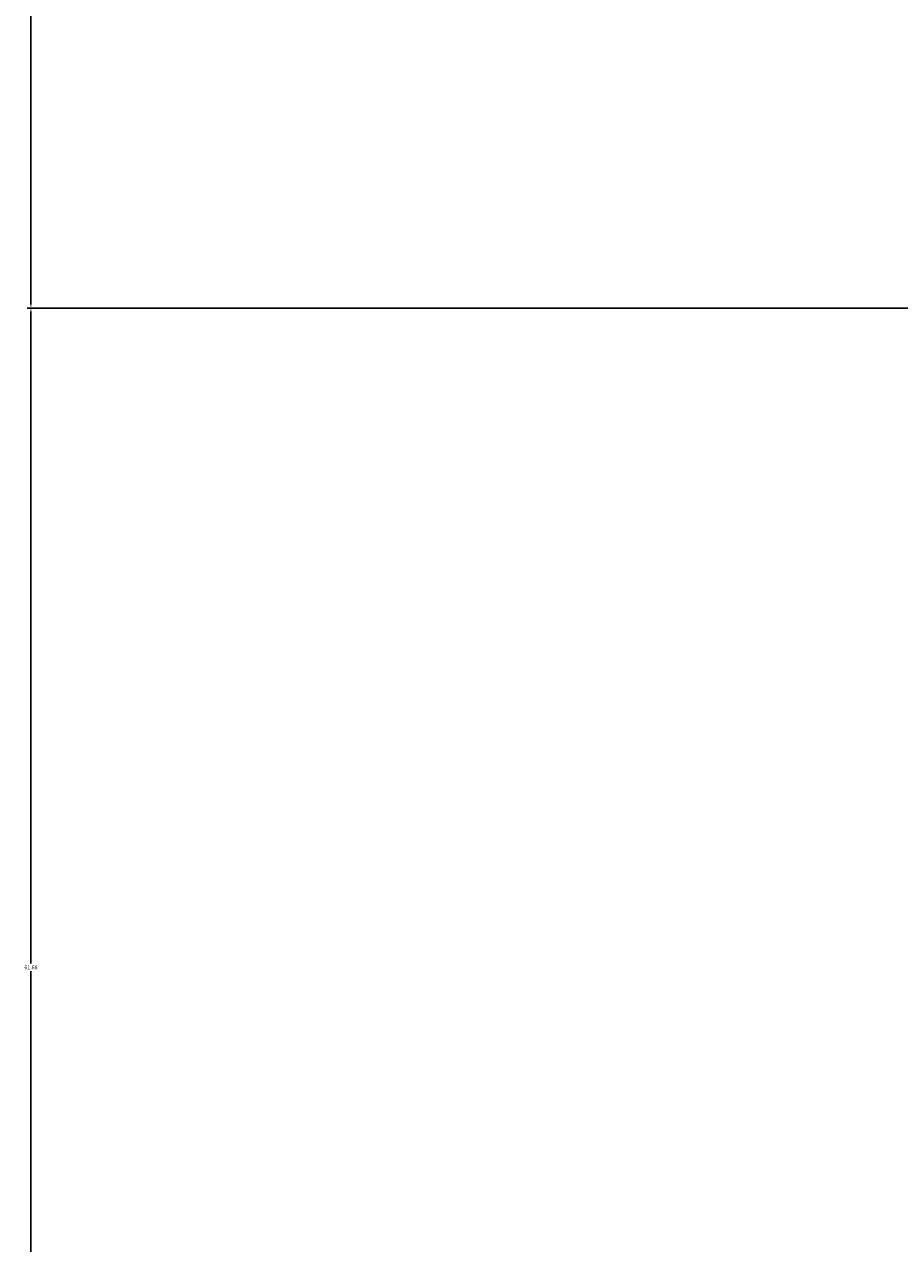
# Model space of a CAD drawing. Units: inches. Extents: x 738 to 1068, y 378 to 757.
# Tile 23 of 41: x 738 to 779, y 549 to 606. Entities that reach past the tile are written whole.
import ezdxf

# ---------------------------------------------------------------- set-up
doc = ezdxf.new("R2010")
doc.units = ezdxf.units.IN
doc.header["$MEASUREMENT"] = 0
doc.layers.add('A-ANNO-DIMS', color=2, linetype='Continuous', lineweight=18)
doc.styles.get("Standard").update_dxf_attribs({"font": 'arial.ttf'})
doc.dimstyles.get("Standard").update_dxf_attribs({"dimtxt": 0.18, "dimasz": 0.18, "dimexe": 0.18, "dimexo": 0.0625, "dimgap": 0.09, "dimtad": 0, "dimtih": 1, "dimtoh": 1, "dimdec": 4, "dimzin": 0, "dimdsep": 46, "dimtxsty": 'Standard', "dimcen": 0.09, "dimadec": 0, "dimazin": 0, "dimtfac": 1, "dimtdec": 4, "dimtofl": 0, "dimtmove": 0, "dimatfit": 3, "dimfxl": 1, "dimtolj": 1, "dimtzin": 0, "dimarcsym": 0})

# ---------------------------------------------------------------- blocks, each defined once
blk = doc.blocks.new('*D22')
at = {"layer": 'A-ANNO-DIMS', "color": 0, "lineweight": -2, "transparency": 16777216}
for p, q in [((781.422, 593.08), (738.194, 593.08)), ((738.374, 592.9), (738.374, 562.422)), ((738.374, 531.581), (738.374, 562.058)), ((781.427, 531.401), (738.194, 531.401))]:
    blk.add_line(p, q, dxfattribs=at)
at = {"layer": 'A-ANNO-DIMS', "color": 0, "transparency": 16777216}
for points in [[(738.344, 592.9), (738.404, 592.9), (738.374, 593.08)], [(738.344, 531.581), (738.404, 531.581), (738.374, 531.401)]]:
    blk.add_solid(points, dxfattribs=at)
at = {"layer": 'Defpoints', "color": 0, "transparency": 16777216}
for p in [(738.374, 593.08), (781.485, 593.08), (781.49, 531.401)]:
    blk.add_point(p, dxfattribs=at)
at = {"layer": 'A-ANNO-DIMS', "color": 0, "transparency": 16777216, "insert": (738.374, 562.24), "char_height": 0.18, "attachment_point": 5}
blk.add_mtext('\\A1;61.68', dxfattribs=at)
blk = doc.blocks.new('*D23')
at = {"layer": 'A-ANNO-DIMS', "color": 0, "lineweight": -2, "transparency": 16777216}
for p, q in [((781.427, 646.985), (738.194, 646.985)), ((738.374, 646.805), (738.374, 620.214)), ((738.374, 593.26), (738.374, 619.85)), ((781.422, 593.08), (738.194, 593.08))]:
    blk.add_line(p, q, dxfattribs=at)
at = {"layer": 'A-ANNO-DIMS', "color": 0, "transparency": 16777216}
for points in [[(738.344, 646.805), (738.404, 646.805), (738.374, 646.985)], [(738.344, 593.26), (738.404, 593.26), (738.374, 593.08)]]:
    blk.add_solid(points, dxfattribs=at)
at = {"layer": 'Defpoints', "color": 0, "transparency": 16777216}
for p in [(738.374, 646.985), (781.49, 646.985), (781.485, 593.08)]:
    blk.add_point(p, dxfattribs=at)
at = {"layer": 'A-ANNO-DIMS', "color": 0, "transparency": 16777216, "insert": (738.374, 620.032), "char_height": 0.18, "attachment_point": 5}
blk.add_mtext('\\A1;53.91', dxfattribs=at)

msp = doc.modelspace()

# ---------------------------------------------------------------- dimensions: what is measured, and where the dimension line sits
at = {"layer": 'A-ANNO-DIMS'}
for base, p1, p2, picture, middle in [((738.3736, 646.9853), (781.4846, 593.0796), (781.4897, 646.9853), '*D23', (738.3736, 620.0325)), ((738.3736, 593.0796), (781.4897, 531.4009), (781.4846, 593.0796), '*D22', (738.3736, 562.2403))]:
    dim = msp.add_linear_dim(base=base, p1=p1, p2=p2, angle=90, dimstyle='Standard', override={"dimdec": 2, "dimlfac": 1, "dimrnd": 0, "dimzin": 0, "dimdsep": 46, "dimlunit": 2}, dxfattribs=at)
    dim.commit()
    dim.dimension.update_dxf_attribs({"geometry": picture, "text_midpoint": middle})

doc.saveas('drawing.dxf')
